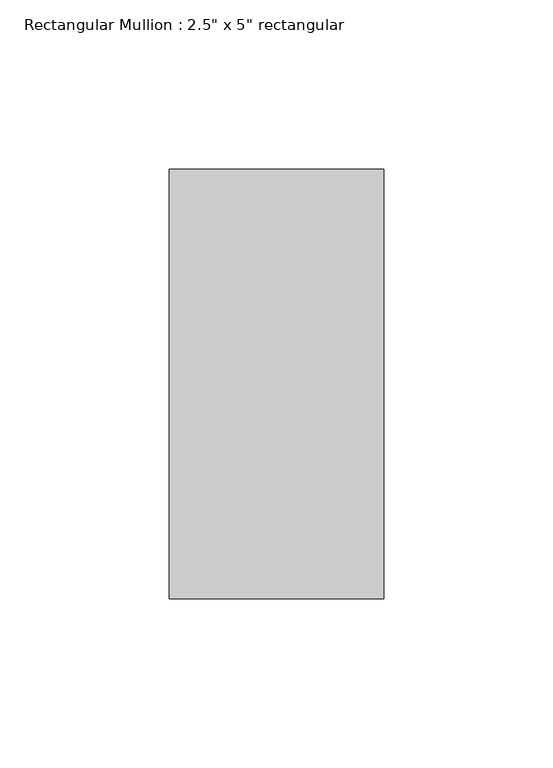
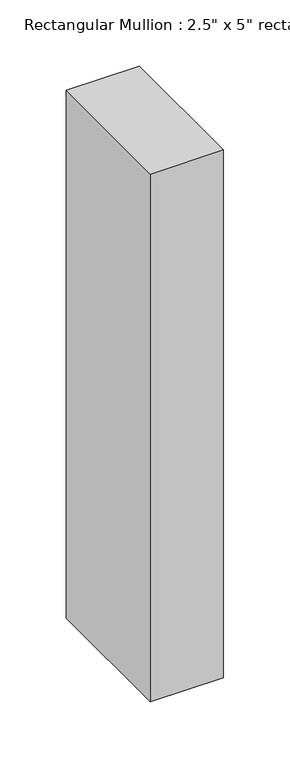
"""IFC4 building model written with IfcOpenShell, lengths in millimetres: member geometry."""

from ifc_helpers import new_model, si_unit, frame, origin, place, context, project, spatial, polyline, outline, extrude, source, transform, mapped, element, save


def member_499db0bc(model_context):
    return source(origin(), model_context, "Body", "SweptSolid", [
        extrude(outline(polyline([(0.0, 63.5), (0.0, -63.5), (-63.5, -63.5), (-63.5, 63.5), (0.0, 63.5)])), frame((0.0, 0.0, -485.8142755), z_axis=(0.0, 0.0, 1.0), x_axis=(1.0, 0.0, 0.0)), (0.0, 0.0, 1.0), 485.8142755),
    ])


if __name__ == "__main__":
    model = new_model("IFC4")
    model_context = context("Model", 3, world=origin())
    ifc_project = project(units=[si_unit("LENGTHUNIT", "METRE", prefix="MILLI")], contexts=[model_context])
    site = spatial("IfcSite", under=ifc_project)
    building = spatial("IfcBuilding", under=site)
    placement = place(None, origin())
    member_shape = member_499db0bc(model_context)
    element("IfcMember", 1, ObjectType="Rectangular Mullion : 2.5\" x 5\" rectangular", at=placement, inside=building, context=model_context, shape_type="MappedRepresentation", body=[
        mapped(member_shape, transform((0.0, 0.0, 0.0), x_axis=(1.0, 0.0, 0.0), y_axis=(0.0, 1.0, 0.0), z_axis=(0.0, 0.0, 1.0))),
    ])
    save(model, "model.ifc")

# Revit data of these elements
# Type "Rectangular Mullion : 2.5\" x 5\" rectangular"
#   built-in parameter 1007304 = 0.416667 (stored number, unit not read)
#   built-in parameter 1007301 = 0.104167 (stored number, unit not read)
#   built-in parameter 1007300 = 0.104167 (stored number, unit not read)
# Element 1 (IfcMember, "Rectangular Mullion : 2.5\" x 5\" rectangular")
#   Materials on its faces: "Aluminum"
# Materials
#   "Aluminum": class "Metal", colour RGB 247 247 247, transparency 0, Description = "Aluminum 6061", Cost = 0
